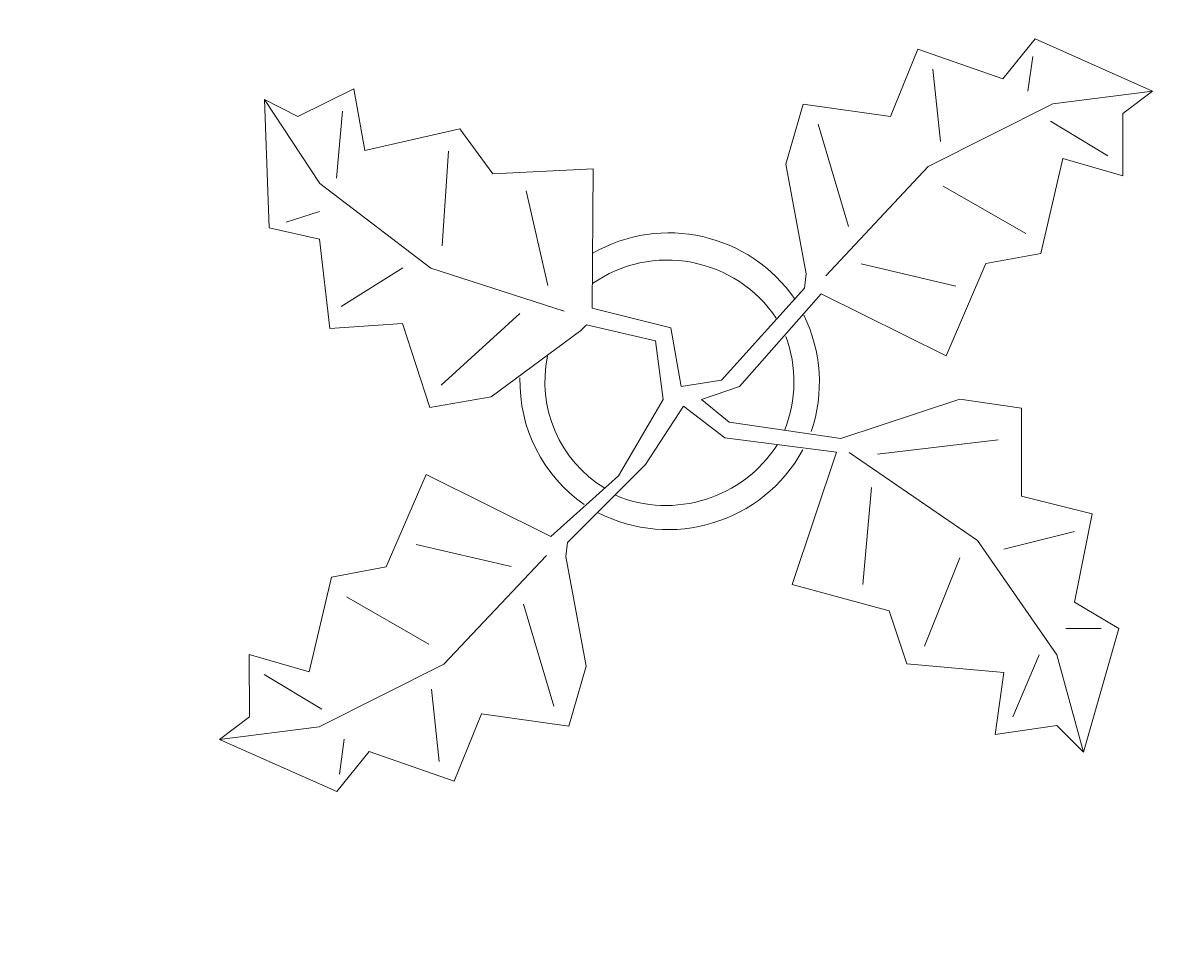
# Model space of a CAD drawing. Units: inches. Extents: x -301 to 715, y -607 to 364.
# Tile 62 of 141: x -93 to -62, y -260 to -235. Entities that reach past the tile are written whole.
import ezdxf

# ---------------------------------------------------------------- set-up
doc = ezdxf.new("R2010")
doc.units = ezdxf.units.IN
doc.header["$MEASUREMENT"] = 0
doc.layers.add('A-ANNO-DIMS', color=2, linetype='Continuous', lineweight=18)
doc.layers.add('L-PLNT', color=94, linetype='Continuous', lineweight=13)
doc.styles.get("Standard").update_dxf_attribs({"font": 'arial.ttf'})
doc.dimstyles.get("Standard").update_dxf_attribs({"dimtxt": 0.18, "dimasz": 0.18, "dimexe": 0.18, "dimexo": 0.0625, "dimgap": 0.09, "dimtad": 0, "dimtih": 1, "dimtoh": 1, "dimdec": 1, "dimzin": 0, "dimdsep": 46, "dimlunit": 4, "dimtxsty": 'Standard', "dimcen": 0.09, "dimclrd": 3, "dimclre": 4, "dimclrt": 6, "dimadec": 0, "dimazin": 0, "dimtfac": 1, "dimtdec": 1, "dimtofl": 0, "dimtmove": 0, "dimatfit": 3, "dimfxl": 1, "dimtfill": 2, "dimtfillclr": 51, "dimtolj": 1, "dimtzin": 0, "dimarcsym": 0})

# ---------------------------------------------------------------- blocks, each defined once
blk = doc.blocks.new('Plant - Rubber or Philodendron')
for p, q in [((13.3837, 12.301), (14.68, 13.9039)), ((14.68, 13.9039), (19.3848, 11.8146)), ((8.8871, 10.7908), (9.9809, 13.4933)), ((9.9809, 13.4933), (13.3837, 12.301)), ((14.5816, 13.2037), (14.3848, 11.8033)), ((10.5828, 12.6946), (10.8893, 9.7953)), ((-14.8639, 10.7964), (-12.6195, 11.8975)), ((-12.6195, 11.8975), (-12.1909, 9.4345)), ((19.3848, 11.8146), (15.3859, 11.3055)), ((19.3848, 11.8146), (18.1868, 10.9119)), ((-16.2005, 11.4774), (-13.9899, 8.1064)), ((-16.2005, 11.4774), (-14.8639, 10.7964)), ((-16.0159, 6.3329), (-16.2005, 11.4774)), ((4.6914, 8.8812), (5.3859, 11.2828)), ((5.3859, 11.2828), (8.8871, 10.7908)), ((15.3859, 11.3055), (10.3916, 8.7942)), ((-13.3174, 8.325), (-13.0735, 11.0065)), ((15.2875, 10.6053), (17.5907, 9.2105)), ((18.1868, 10.9119), (18.1925, 8.4119)), ((-12.1909, 9.4345), (-8.3829, 10.3)), ((-8.3829, 10.3), (-7.0549, 8.501)), ((5.9878, 10.4842), (7.1971, 6.3869)), ((-8.8369, 9.409), (-9.0894, 5.6095)), ((4.6914, 8.8812), (5.5014, 4.4831)), ((10.3916, 8.7942), (6.2847, 4.4028)), ((15.7909, 9.1065), (14.8995, 5.3044)), ((18.1925, 8.4119), (15.7909, 9.1065)), ((-7.0549, 8.501), (-3.0284, 8.6941)), ((-3.0284, 8.6941), (-3.0709, 3.1041)), ((-13.9899, 8.1064), (-9.5434, 4.7185)), ((14.2977, 6.1031), (10.9934, 7.9956)), ((-4.8529, 4.012), (-5.7184, 7.82)), ((-15.3434, 6.5514), (-13.9984, 6.9884)), ((-14.0069, 5.8704), (-16.0159, 6.3329)), ((-13.5868, 2.2894), (-14.0069, 5.8704)), ((14.8995, 5.3044), (12.7005, 4.8994)), ((-13.1329, 3.1804), (-10.6614, 4.727)), ((-9.5434, 4.7185), (-4.1917, 2.9888)), ((7.7005, 4.8881), (11.5025, 3.9967)), ((12.7005, 4.8994), (11.1089, 1.1958)), ((5.4346, 3.9146), (5.5014, 4.4831)), ((2.1141, 0.2298), (5.4346, 3.9146)), ((6.1032, 3.6844), (2.8262, -0.031)), ((11.1089, 1.1958), (6.1032, 3.6844)), ((-9.1318, 0.0195), (-5.9793, 2.9025)), ((-3.0709, 3.1041), (0.0797, 2.3163)), ((-10.6784, 2.491), (-13.5868, 2.2894)), ((-9.5858, -0.8715), (-10.6784, 2.491)), ((-3.5248, 2.2131), (-3.3011, 2.4355)), ((-3.3011, 2.4355), (-0.5306, 1.7947)), ((0.0797, 2.3163), (0.4866, -0.031)), ((-7.1228, -0.443), (-3.5248, 2.2131)), ((-0.5306, 1.7947), (-0.2255, -0.5527)), ((-0.5306, 1.7947), (-0.5306, 1.7947)), ((0.4866, -0.031), (2.1141, 0.2298)), ((-7.1228, -0.443), (-9.5858, -0.8715)), ((2.8262, -0.031), (1.3003, -0.5527)), ((-2.019, -3.6148), (-0.2255, -0.5527)), ((-0.9375, -3.1608), (0.5883, -0.8135)), ((0.5883, -0.8135), (2.2447, -2.0916)), ((1.3003, -0.5527), (2.4193, -1.4655)), ((11.6605, -0.5413), (6.895, -2.1175)), ((11.6605, -0.5413), (14.1354, -0.8948)), ((14.1354, -0.8948), (14.1354, -4.4304)), ((2.4193, -1.4655), (6.895, -2.1175)), ((2.2447, -2.0916), (6.7108, -2.6626)), ((8.3544, -2.7453), (13.1973, -2.1704)), ((4.943, -7.9659), (6.7108, -2.6626)), ((12.3677, -6.1981), (7.219, -2.6772)), ((-4.0579, -6.2781), (-0.9375, -3.1608)), ((-11.3237, -7.2629), (-9.7321, -3.5593)), ((-9.7321, -3.5593), (-4.7264, -6.0479)), ((-2.019, -3.6148), (-4.7264, -6.0479)), ((8.125, -4.0768), (7.7715, -7.9659)), ((14.1354, -4.4304), (16.9638, -5.1375)), ((16.9638, -5.1375), (16.2567, -8.673)), ((16.2567, -5.8446), (13.4283, -6.5517)), ((-6.3237, -7.2516), (-10.1257, -6.3602)), ((-4.1246, -6.8466), (-4.0579, -6.2781)), ((15.5496, -10.7943), (12.3677, -6.1981)), ((-9.0148, -11.1577), (-4.9047, -6.8122)), ((-3.3146, -11.2447), (-4.1246, -6.8466)), ((10.2463, -10.4408), (11.6605, -6.9053)), ((-13.5228, -7.6679), (-11.3237, -7.2629)), ((-14.4141, -11.4699), (-13.5228, -7.6679)), ((8.8321, -9.0266), (4.943, -7.9659)), ((-12.921, -8.4665), (-9.6166, -10.359)), ((-4.611, -12.8477), (-5.8203, -8.7504)), ((16.2567, -8.673), (18.0245, -9.7337)), ((9.5392, -11.1479), (8.8321, -9.0266)), ((17.3174, -9.7337), (15.9032, -9.7337)), ((18.0245, -9.7337), (16.6103, -14.6834)), ((-16.8157, -10.7754), (-14.4141, -11.4699)), ((-16.8101, -13.2754), (-16.8157, -10.7754)), ((14.8425, -10.7943), (13.7819, -13.2692)), ((16.6103, -14.6834), (15.5496, -10.7943)), ((-14.0091, -13.669), (-9.0148, -11.1577)), ((-3.3146, -11.2447), (-4.0092, -13.6463)), ((13.4283, -11.5015), (9.5392, -11.1479)), ((13.0748, -13.9763), (13.4283, -11.5015)), ((-13.9107, -12.9688), (-16.2139, -11.574)), ((-9.206, -15.0581), (-9.5126, -12.1588)), ((-18.008, -14.1781), (-16.8101, -13.2754)), ((-7.5103, -13.1543), (-8.6042, -15.8568)), ((-4.0092, -13.6463), (-7.5103, -13.1543)), ((-18.008, -14.1781), (-14.0091, -13.669)), ((15.5496, -13.6228), (13.0748, -13.9763)), ((16.6103, -14.6834), (15.5496, -13.6228)), ((-13.3032, -16.2674), (-18.008, -14.1781)), ((-13.2048, -15.5672), (-13.008, -14.1668)), ((-12.0069, -14.6645), (-13.3032, -16.2674)), ((-8.6042, -15.8568), (-12.0069, -14.6645))]:
    blk.add_line(p, q)
for centre, radius, start, end in [((0, 0), 6.1275, 34.37569, 120.1028), ((-0.0601, -0.2075), 5.2461, 33.82192, 124.9414), ((-0.098, 0.1364), 6.1288, 341.2017, 26.09184), ((-0.2664, 0.1682), 5.2775, 338.4094, 20.03007), ((0.0308, 0.1664), 5, 168.1647, 238.6725), ((0.0308, 0.1664), 6, 178.6147, 235.1169), ((-0.0234, 0.3825), 6.1492, 242.5812, 331.2714), ((-0.1102, 0.4886), 5.2883, 247.3711, 327.472)]:
    blk.add_arc(centre, radius, start, end)
blk = doc.blocks.new('*D147')
at = {"layer": 'A-ANNO-DIMS', "color": 4, "lineweight": -2, "transparency": 16777216}
for p, q in [((-103.603, -223.88), (-103.603, -296.865)), ((-45.603, -223.88), (-45.603, -296.865))]:
    blk.add_line(p, q, dxfattribs=at)
at = {"layer": 'A-ANNO-DIMS', "color": 3, "lineweight": -2, "transparency": 16777216}
for p, q in [((-103.423, -296.685), (-75.006, -296.685)), ((-45.783, -296.685), (-74.2, -296.685))]:
    blk.add_line(p, q, dxfattribs=at)
at = {"layer": 'A-ANNO-DIMS', "color": 3, "transparency": 16777216}
for points in [[(-103.423, -296.655), (-103.423, -296.715), (-103.603, -296.685)], [(-45.783, -296.655), (-45.783, -296.715), (-45.603, -296.685)]]:
    blk.add_solid(points, dxfattribs=at)
at = {"layer": 'Defpoints', "color": 0, "transparency": 16777216}
for p in [(-103.603, -223.818), (-45.603, -223.818), (-45.603, -296.685)]:
    blk.add_point(p, dxfattribs=at)
at = {"layer": 'A-ANNO-DIMS', "color": 6, "transparency": 16777216, "insert": (-74.603, -296.685), "char_height": 0.18, "attachment_point": 5, "bg_fill": 1, "box_fill_scale": 1.25, "bg_fill_color": 51, "bg_fill_transparency": 0}
blk.add_mtext('\\A1;4\'-10"', dxfattribs=at)
blk = doc.blocks.new('*D158')
at = {"layer": 'A-ANNO-DIMS', "color": 4, "lineweight": -2, "transparency": 16777216}
for p, q in [((-122.603, 221.62), (-122.603, -296.865)), ((-50.603, 221.62), (-50.603, -296.865))]:
    blk.add_line(p, q, dxfattribs=at)
at = {"layer": 'A-ANNO-DIMS', "color": 3, "lineweight": -2, "transparency": 16777216}
for p, q in [((-122.423, -296.685), (-86.933, -296.685)), ((-50.783, -296.685), (-86.274, -296.685))]:
    blk.add_line(p, q, dxfattribs=at)
at = {"layer": 'A-ANNO-DIMS', "color": 3, "transparency": 16777216}
for points in [[(-122.423, -296.655), (-122.423, -296.715), (-122.603, -296.685)], [(-50.783, -296.655), (-50.783, -296.715), (-50.603, -296.685)]]:
    blk.add_solid(points, dxfattribs=at)
at = {"layer": 'Defpoints', "color": 0, "transparency": 16777216}
for p in [(-122.603, 221.682), (-50.603, 221.682), (-50.603, -296.685)]:
    blk.add_point(p, dxfattribs=at)
at = {"layer": 'A-ANNO-DIMS', "color": 6, "transparency": 16777216, "insert": (-86.603, -296.685), "char_height": 0.18, "attachment_point": 5, "bg_fill": 1, "box_fill_scale": 1.25, "bg_fill_color": 51, "bg_fill_transparency": 0}
blk.add_mtext('\\A1;6\'-0"', dxfattribs=at)

msp = doc.modelspace()

# ---------------------------------------------------------------- block references
at = {"layer": 'L-PLNT', "xscale": 0.6613521884636907, "yscale": 0.6613521884636907, "zscale": 0.6613521884636907}
msp.add_blockref('Plant - Rubber or Philodendron', (-75.535, -244.98), dxfattribs=at)

# ---------------------------------------------------------------- dimensions: what is measured, and where the dimension line sits
at = {"layer": 'A-ANNO-DIMS'}
for base, p1, p2, picture, middle in [((-50.603, -296.685), (-122.603, 221.682), (-50.603, 221.682), '*D158', (-86.603, -296.685)), ((-45.603, -296.685), (-103.603, -223.818), (-45.603, -223.818), '*D147', (-74.603, -296.685))]:
    dim = msp.add_linear_dim(base=base, p1=p1, p2=p2, dimstyle='Standard', override={"dimdec": 1, "dimlfac": 1, "dimrnd": 0, "dimzin": 1, "dimdsep": 46, "dimlunit": 4, "dimfrac": 2}, dxfattribs=at)
    dim.commit()
    dim.dimension.update_dxf_attribs({"geometry": picture, "text_midpoint": middle})

doc.saveas('drawing.dxf')
